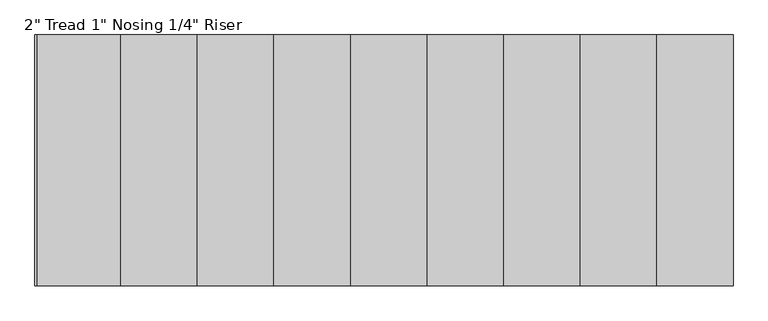
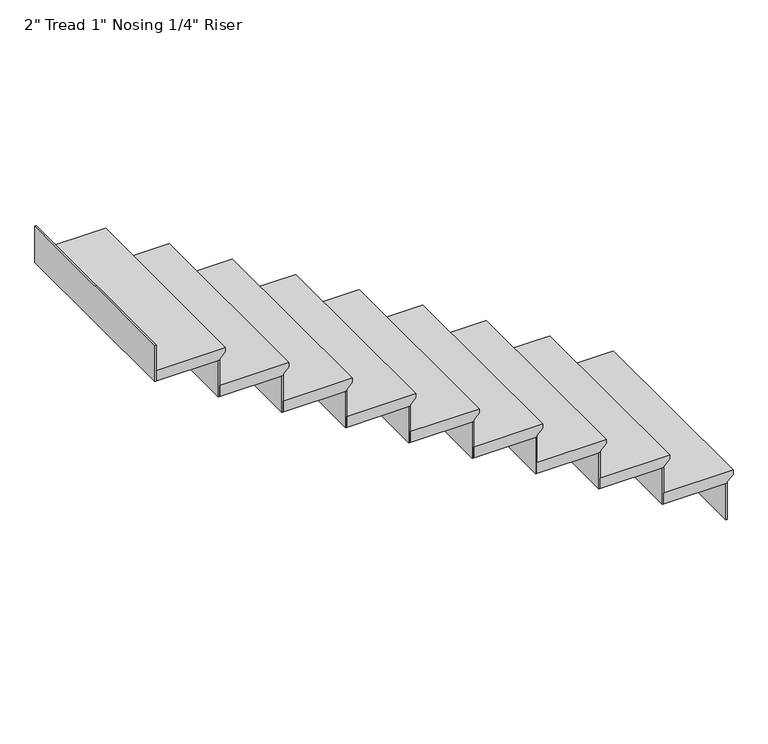
"""IFC4 building model written with IfcOpenShell, lengths in millimetres: stair flight geometry."""

from ifc_helpers import new_model, si_unit, frame, origin, place, context, project, spatial, polyline, outline, extrude, source, transform, mapped, element, save


def stair_flight_e67f926d(model_context):
    return source(origin(), model_context, "Body", "SweptSolid", [
        extrude(outline(polyline([(1524.0, -1680.9866603), (1524.0, -1985.7866603), (1473.2, -1985.7866603), (1473.2, -1706.3866603), (1479.55, -1706.3866603), (1504.95, -1680.9866603), (1524.0, -1680.9866603)])), frame((0.0, -4415.5331121, 0.0), z_axis=(0.0, 1.0, 0.0), x_axis=(0.0, 0.0, 1.0)), (0.0, 0.0, 1.0), 914.4),
        extrude(outline(polyline([(-1712.7366603, -3501.1331121), (-1706.3866603, -3501.1331121), (-1706.3866603, -4415.5331121), (-1712.7366603, -4415.5331121), (-1712.7366603, -3501.1331121)])), frame((0.0, 0.0, 1303.8666667), z_axis=(0.0, 0.0, 1.0), x_axis=(1.0, 0.0, 0.0)), (0.0, 0.0, 1.0), 169.3333333),
        extrude(outline(polyline([(-1992.1366603, -3501.1331121), (-1985.7866603, -3501.1331121), (-1985.7866603, -4415.5331121), (-1992.1366603, -4415.5331121), (-1992.1366603, -3501.1331121)])), frame((0.0, 0.0, 1473.2), z_axis=(0.0, 0.0, 1.0), x_axis=(1.0, 0.0, 0.0)), (0.0, 0.0, 1.0), 169.3333333),
        extrude(outline(polyline([(1693.3333333, -1960.3866603), (1693.3333333, -2265.1866603), (1642.5333333, -2265.1866603), (1642.5333333, -1985.7866603), (1648.8833333, -1985.7866603), (1674.2833333, -1960.3866603), (1693.3333333, -1960.3866603)])), frame((0.0, -4415.5331121, 0.0), z_axis=(0.0, 1.0, 0.0), x_axis=(0.0, 0.0, 1.0)), (0.0, 0.0, 1.0), 914.4),
        extrude(outline(polyline([(-2271.5366603, -3501.1331121), (-2265.1866603, -3501.1331121), (-2265.1866603, -4415.5331121), (-2271.5366603, -4415.5331121), (-2271.5366603, -3501.1331121)])), frame((0.0, 0.0, 1642.5333333), z_axis=(0.0, 0.0, 1.0), x_axis=(1.0, 0.0, 0.0)), (0.0, 0.0, 1.0), 169.3333333),
        extrude(outline(polyline([(1862.6666667, -2239.7866603), (1862.6666667, -2544.5866603), (1811.8666667, -2544.5866603), (1811.8666667, -2265.1866603), (1818.2166667, -2265.1866603), (1843.6166667, -2239.7866603), (1862.6666667, -2239.7866603)])), frame((0.0, -4415.5331121, 0.0), z_axis=(0.0, 1.0, 0.0), x_axis=(0.0, 0.0, 1.0)), (0.0, 0.0, 1.0), 914.4),
        extrude(outline(polyline([(-2550.9366603, -3501.1331121), (-2544.5866603, -3501.1331121), (-2544.5866603, -4415.5331121), (-2550.9366603, -4415.5331121), (-2550.9366603, -3501.1331121)])), frame((0.0, 0.0, 1811.8666667), z_axis=(0.0, 0.0, 1.0), x_axis=(1.0, 0.0, 0.0)), (0.0, 0.0, 1.0), 169.3333333),
        extrude(outline(polyline([(2032.0, -2519.1866603), (2032.0, -2823.9866603), (1981.2, -2823.9866603), (1981.2, -2544.5866603), (1987.55, -2544.5866603), (2012.95, -2519.1866603), (2032.0, -2519.1866603)])), frame((0.0, -4415.5331121, 0.0), z_axis=(0.0, 1.0, 0.0), x_axis=(0.0, 0.0, 1.0)), (0.0, 0.0, 1.0), 914.4),
        extrude(outline(polyline([(-2830.3366603, -3501.1331121), (-2823.9866603, -3501.1331121), (-2823.9866603, -4415.5331121), (-2830.3366603, -4415.5331121), (-2830.3366603, -3501.1331121)])), frame((0.0, 0.0, 1981.2), z_axis=(0.0, 0.0, 1.0), x_axis=(1.0, 0.0, 0.0)), (0.0, 0.0, 1.0), 169.3333333),
        extrude(outline(polyline([(2201.3333333, -2798.5866603), (2201.3333333, -3103.3866603), (2150.5333333, -3103.3866603), (2150.5333333, -2823.9866603), (2156.8833333, -2823.9866603), (2182.2833333, -2798.5866603), (2201.3333333, -2798.5866603)])), frame((0.0, -4415.5331121, 0.0), z_axis=(0.0, 1.0, 0.0), x_axis=(0.0, 0.0, 1.0)), (0.0, 0.0, 1.0), 914.4),
        extrude(outline(polyline([(-3109.7366603, -3501.1331121), (-3103.3866603, -3501.1331121), (-3103.3866603, -4415.5331121), (-3109.7366603, -4415.5331121), (-3109.7366603, -3501.1331121)])), frame((0.0, 0.0, 2150.5333333), z_axis=(0.0, 0.0, 1.0), x_axis=(1.0, 0.0, 0.0)), (0.0, 0.0, 1.0), 169.3333333),
        extrude(outline(polyline([(2370.6666667, -3077.9866603), (2370.6666667, -3382.7866603), (2319.8666667, -3382.7866603), (2319.8666667, -3103.3866603), (2326.2166667, -3103.3866603), (2351.6166667, -3077.9866603), (2370.6666667, -3077.9866603)])), frame((0.0, -4415.5331121, 0.0), z_axis=(0.0, 1.0, 0.0), x_axis=(0.0, 0.0, 1.0)), (0.0, 0.0, 1.0), 914.4),
        extrude(outline(polyline([(-3389.1366603, -3501.1331121), (-3382.7866603, -3501.1331121), (-3382.7866603, -4415.5331121), (-3389.1366603, -4415.5331121), (-3389.1366603, -3501.1331121)])), frame((0.0, 0.0, 2319.8666667), z_axis=(0.0, 0.0, 1.0), x_axis=(1.0, 0.0, 0.0)), (0.0, 0.0, 1.0), 169.3333333),
        extrude(outline(polyline([(2540.0, -3357.3866603), (2540.0, -3662.1866603), (2489.2, -3662.1866603), (2489.2, -3382.7866603), (2495.55, -3382.7866603), (2520.95, -3357.3866603), (2540.0, -3357.3866603)])), frame((0.0, -4415.5331121, 0.0), z_axis=(0.0, 1.0, 0.0), x_axis=(0.0, 0.0, 1.0)), (0.0, 0.0, 1.0), 914.4),
        extrude(outline(polyline([(-3668.5366603, -3501.1331121), (-3662.1866603, -3501.1331121), (-3662.1866603, -4415.5331121), (-3668.5366603, -4415.5331121), (-3668.5366603, -3501.1331121)])), frame((0.0, 0.0, 2489.2), z_axis=(0.0, 0.0, 1.0), x_axis=(1.0, 0.0, 0.0)), (0.0, 0.0, 1.0), 169.3333333),
        extrude(outline(polyline([(2709.3333333, -3636.7866603), (2709.3333333, -3941.5866603), (2658.5333333, -3941.5866603), (2658.5333333, -3662.1866603), (2664.8833333, -3662.1866603), (2690.2833333, -3636.7866603), (2709.3333333, -3636.7866603)])), frame((0.0, -4415.5331121, 0.0), z_axis=(0.0, 1.0, 0.0), x_axis=(0.0, 0.0, 1.0)), (0.0, 0.0, 1.0), 914.4),
        extrude(outline(polyline([(-3947.9366603, -3501.1331121), (-3941.5866603, -3501.1331121), (-3941.5866603, -4415.5331121), (-3947.9366603, -4415.5331121), (-3947.9366603, -3501.1331121)])), frame((0.0, 0.0, 2658.5333333), z_axis=(0.0, 0.0, 1.0), x_axis=(1.0, 0.0, 0.0)), (0.0, 0.0, 1.0), 169.3333333),
        extrude(outline(polyline([(-4227.3366603, -3501.1331121), (-4220.9866603, -3501.1331121), (-4220.9866603, -4415.5331121), (-4227.3366603, -4415.5331121), (-4227.3366603, -3501.1331121)])), frame((0.0, 0.0, 2827.8666667), z_axis=(0.0, 0.0, 1.0), x_axis=(1.0, 0.0, 0.0)), (0.0, 0.0, 1.0), 169.3333333),
        extrude(outline(polyline([(2878.6666667, -3916.1866603), (2878.6666667, -4220.9866603), (2827.8666667, -4220.9866603), (2827.8666667, -3941.5866603), (2834.2166667, -3941.5866603), (2859.6166667, -3916.1866603), (2878.6666667, -3916.1866603)])), frame((0.0, -4415.5331121, 0.0), z_axis=(0.0, 1.0, 0.0), x_axis=(0.0, 0.0, 1.0)), (0.0, 0.0, 1.0), 914.4),
    ])


if __name__ == "__main__":
    model = new_model("IFC4")
    model_context = context("Model", 3, world=origin())
    ifc_project = project(units=[si_unit("LENGTHUNIT", "METRE", prefix="MILLI")], contexts=[model_context])
    site = spatial("IfcSite", under=ifc_project)
    building = spatial("IfcBuilding", under=site)
    placement = place(None, origin())
    stair_flight_shape = stair_flight_e67f926d(model_context)
    element("IfcStairFlight", 1, ObjectType="2\" Tread 1\" Nosing 1/4\" Riser", at=placement, inside=building, context=model_context, shape_type="MappedRepresentation", body=[
        mapped(stair_flight_shape, transform((0.0, 0.0, 0.0), x_axis=(1.0, 0.0, 0.0), y_axis=(0.0, 1.0, 0.0), z_axis=(0.0, 0.0, 1.0))),
    ])
    save(model, "model.ifc")
